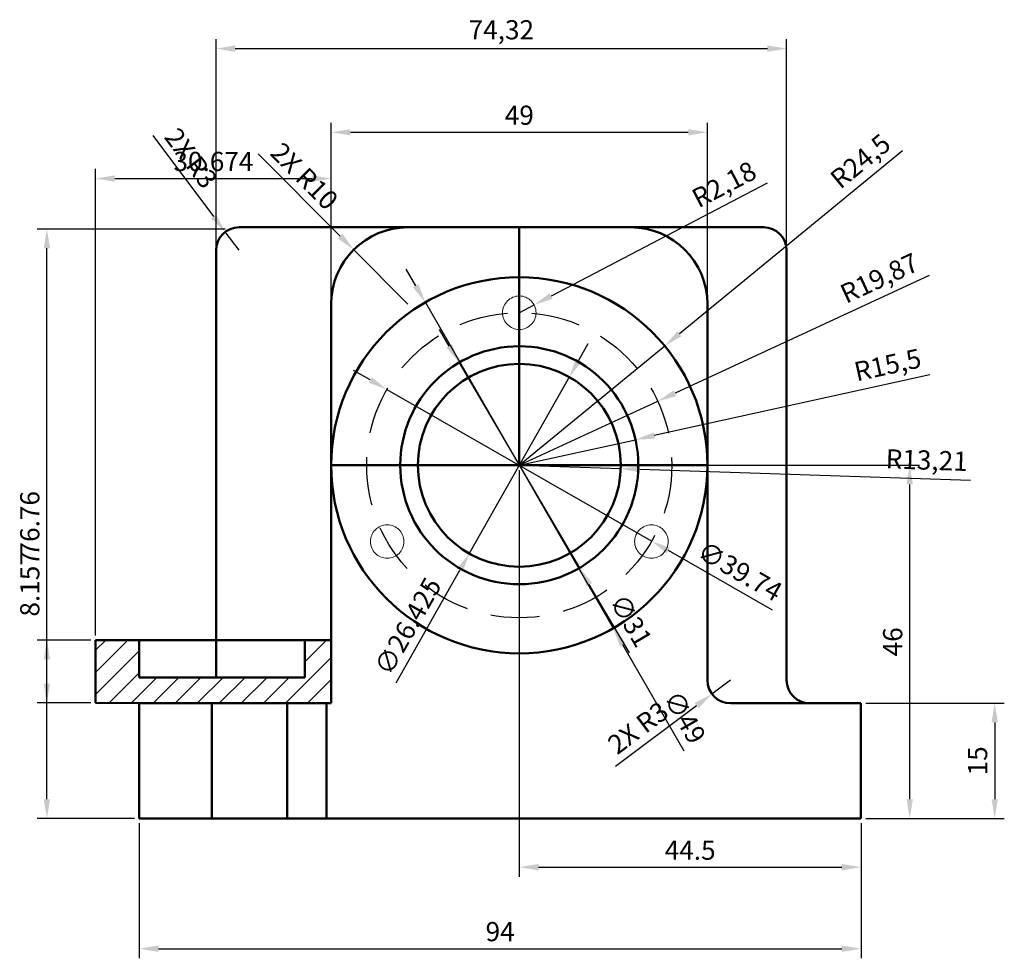
# Model space of a CAD drawing. Units: millimetres. Extents: x 1381 to 2009, y 1325 to 1613.
# Tile 5 of 6: x 1622 to 1750, y 1491 to 1613. Entities that reach past the tile are written whole.
import ezdxf

# ---------------------------------------------------------------- set-up
doc = ezdxf.new("R2010")
doc.units = ezdxf.units.MM
doc.linetypes.add('CENTER', pattern=[50.8, 31.75, -6.35, 6.35, -6.35])
doc.linetypes.add('HIDDEN', pattern=[9.525, 6.35, -3.175])
for name, color, linetype, lineweight in [('M-CNTR', 1, 'CENTER', 18), ('M-DIMS', 2, 'Continuous', 25), ('M-HATC', 8, 'Continuous', 18), ('M-HIDN', 6, 'HIDDEN', 25), ('M-OUTL', 7, 'Continuous', 50)]:
    doc.layers.add(name, color=color, linetype=linetype, lineweight=lineweight)
doc.styles.get("Standard").update_dxf_attribs({"font": 'arial.ttf'})
doc.dimstyles.new('ISO-25', dxfattribs={"dimtxt": 2.5, "dimasz": 2.5, "dimexe": 1.25, "dimexo": 0.625, "dimtad": 1, "dimtxsty": 'Standard', "dimcen": 2.5, "dimadec": 0, "dimazin": 0, "dimtfac": 1, "dimtmove": 0, "dimatfit": 3, "dimfxl": 1, "dimarcsym": 0})

# ---------------------------------------------------------------- blocks, each defined once
blk = doc.blocks.new('*U10')
blk.add_circle((0, 0), 2.18)
blk = doc.blocks.new('*U11')
at = {"layer": 'M-CNTR', "color": 0, "linetype": 'ByBlock', "lineweight": -2, "transparency": 16777216}
blk.add_blockref('*U10', (1686.87, 1575.09), dxfattribs=at)
for p, rotation in [((1669.66, 1545.28), 120), ((1704.07, 1545.28), 240)]:
    blk.add_blockref('*U10', p, dxfattribs=dict(at, rotation=rotation))
blk = doc.blocks.new('*D59')
at = {"layer": 'Defpoints', "color": 0, "transparency": 16777216}
for p in [(1637.37, 1509.22), (1731.37, 1509.22), (1731.37, 1492.25)]:
    blk.add_point(p, dxfattribs=at)
at = {"layer": 'M-DIMS', "color": 0, "lineweight": -2, "transparency": 16777216}
for p, q in [((1637.37, 1508.59), (1637.37, 1491)), ((1731.37, 1508.59), (1731.37, 1491)), ((1639.87, 1492.25), (1728.87, 1492.25))]:
    blk.add_line(p, q, dxfattribs=at)
at = {"layer": 'M-DIMS', "color": 0, "transparency": 16777216}
for points in [[(1639.87, 1492.67), (1639.87, 1491.83), (1637.37, 1492.25)], [(1728.87, 1492.67), (1728.87, 1491.83), (1731.37, 1492.25)]]:
    blk.add_solid(points, dxfattribs=at)
at = {"layer": 'M-DIMS', "color": 0, "transparency": 16777216, "insert": (1684.37, 1494.15), "char_height": 2.5, "attachment_point": 5}
blk.add_mtext('94', dxfattribs=at)
blk = doc.blocks.new('*D60')
at = {"layer": 'Defpoints', "color": 0, "transparency": 16777216}
for p in [(1731.37, 1524.22), (1731.37, 1509.22), (1748.78, 1509.22)]:
    blk.add_point(p, dxfattribs=at)
at = {"layer": 'M-DIMS', "color": 0, "lineweight": -2, "transparency": 16777216}
for p, q in [((1731.99, 1524.22), (1750.03, 1524.22)), ((1748.78, 1521.72), (1748.78, 1511.72)), ((1731.99, 1509.22), (1750.03, 1509.22))]:
    blk.add_line(p, q, dxfattribs=at)
at = {"layer": 'M-DIMS', "color": 0, "transparency": 16777216}
for points in [[(1748.37, 1521.72), (1749.2, 1521.72), (1748.78, 1524.22)], [(1748.37, 1511.72), (1749.2, 1511.72), (1748.78, 1509.22)]]:
    blk.add_solid(points, dxfattribs=at)
at = {"layer": 'M-DIMS', "color": 0, "transparency": 16777216, "insert": (1746.88, 1516.72), "char_height": 2.5, "attachment_point": 5, "rotation": 90}
blk.add_mtext('15', dxfattribs=at)
blk = doc.blocks.new('*D61')
at = {"layer": 'Defpoints', "color": 0, "transparency": 16777216}
for p in [(1721.68, 1609.49), (1647.37, 1583.22), (1721.68, 1583.22)]:
    blk.add_point(p, dxfattribs=at)
at = {"layer": 'M-DIMS', "color": 0, "lineweight": -2, "transparency": 16777216}
for p, q in [((1647.37, 1583.84), (1647.37, 1610.74)), ((1721.68, 1583.84), (1721.68, 1610.74)), ((1649.87, 1609.49), (1719.18, 1609.49))]:
    blk.add_line(p, q, dxfattribs=at)
at = {"layer": 'M-DIMS', "color": 0, "transparency": 16777216}
for points in [[(1649.87, 1609.91), (1649.87, 1609.07), (1647.37, 1609.49)], [(1719.18, 1609.91), (1719.18, 1609.07), (1721.68, 1609.49)]]:
    blk.add_solid(points, dxfattribs=at)
at = {"layer": 'M-DIMS', "color": 0, "transparency": 16777216, "insert": (1684.53, 1611.62), "char_height": 2.5, "attachment_point": 5}
blk.add_mtext('74,32', dxfattribs=at)
blk = doc.blocks.new('*D62')
at = {"layer": 'Defpoints', "color": 0, "transparency": 16777216}
for p in [(1711.37, 1598.59), (1662.37, 1576.22), (1711.37, 1576.22)]:
    blk.add_point(p, dxfattribs=at)
at = {"layer": 'M-DIMS', "color": 0, "lineweight": -2, "transparency": 16777216}
for p, q in [((1662.37, 1576.84), (1662.37, 1599.84)), ((1711.37, 1576.84), (1711.37, 1599.84)), ((1664.87, 1598.59), (1708.87, 1598.59))]:
    blk.add_line(p, q, dxfattribs=at)
at = {"layer": 'M-DIMS', "color": 0, "transparency": 16777216}
for points in [[(1664.87, 1599.01), (1664.87, 1598.18), (1662.37, 1598.59)], [(1708.87, 1599.01), (1708.87, 1598.18), (1711.37, 1598.59)]]:
    blk.add_solid(points, dxfattribs=at)
at = {"layer": 'M-DIMS', "color": 0, "transparency": 16777216, "insert": (1686.87, 1600.49), "char_height": 2.5, "attachment_point": 5}
blk.add_mtext('49', dxfattribs=at)
blk = doc.blocks.new('*D63')
at = {"layer": 'Defpoints', "color": 0, "transparency": 16777216}
for p in [(1705.8, 1570.76), (1686.87, 1555.22)]:
    blk.add_point(p, dxfattribs=at)
at = {"layer": 'M-DIMS', "color": 0, "lineweight": -2, "transparency": 16777216}
for p, q in [((1736.76, 1596.17), (1707.74, 1572.35)), ((1686.87, 1555.22), (1705.8, 1570.76))]:
    blk.add_line(p, q, dxfattribs=at)
at = {"layer": 'M-DIMS', "color": 0, "transparency": 16777216}
blk.add_solid([(1707.47, 1572.67), (1708, 1572.03), (1705.8, 1570.76)], dxfattribs=at)
at = {"layer": 'M-DIMS', "color": 0, "transparency": 16777216, "insert": (1731.49, 1594.59), "char_height": 2.5, "attachment_point": 5, "rotation": 39.3795}
blk.add_mtext('R24,5', dxfattribs=at)
blk = doc.blocks.new('*D64')
at = {"layer": 'Defpoints', "color": 0, "transparency": 16777216}
for p in [(1704.9, 1563.56), (1686.87, 1555.22)]:
    blk.add_point(p, dxfattribs=at)
at = {"layer": 'M-DIMS', "color": 0, "lineweight": -2, "transparency": 16777216}
for p, q in [((1740.26, 1579.92), (1707.17, 1564.61)), ((1686.87, 1555.22), (1704.9, 1563.56))]:
    blk.add_line(p, q, dxfattribs=at)
at = {"layer": 'M-DIMS', "color": 0, "transparency": 16777216}
blk.add_solid([(1706.99, 1564.99), (1707.34, 1564.23), (1704.9, 1563.56)], dxfattribs=at)
at = {"layer": 'M-DIMS', "color": 0, "transparency": 16777216, "insert": (1733.89, 1579.31), "char_height": 2.5, "attachment_point": 5, "rotation": 24.8223}
blk.add_mtext('R19,87', dxfattribs=at)
blk = doc.blocks.new('*D65')
at = {"layer": 'Defpoints', "color": 0, "transparency": 16777216}
for p in [(1702, 1558.55), (1686.87, 1555.22)]:
    blk.add_point(p, dxfattribs=at)
at = {"layer": 'M-DIMS', "color": 0, "lineweight": -2, "transparency": 16777216}
for p, q in [((1740.33, 1566.99), (1704.45, 1559.09)), ((1686.87, 1555.22), (1702, 1558.55))]:
    blk.add_line(p, q, dxfattribs=at)
at = {"layer": 'M-DIMS', "color": 0, "transparency": 16777216}
blk.add_solid([(1704.36, 1559.5), (1704.54, 1558.68), (1702, 1558.55)], dxfattribs=at)
at = {"layer": 'M-DIMS', "color": 0, "transparency": 16777216, "insert": (1734.91, 1567.98), "char_height": 2.5, "attachment_point": 5, "rotation": 12.4201}
blk.add_mtext('R15,5', dxfattribs=at)
blk = doc.blocks.new('*D66')
at = {"layer": 'Defpoints', "color": 0, "transparency": 16777216}
for p in [(1686.87, 1555.22), (1700.07, 1554.78)]:
    blk.add_point(p, dxfattribs=at)
at = {"layer": 'M-DIMS', "color": 0, "lineweight": -2, "transparency": 16777216}
for p, q in [((1686.87, 1555.22), (1700.07, 1554.78)), ((1745.64, 1553.25), (1702.57, 1554.69))]:
    blk.add_line(p, q, dxfattribs=at)
at = {"layer": 'M-DIMS', "color": 0, "transparency": 16777216}
blk.add_solid([(1702.59, 1555.11), (1702.56, 1554.28), (1700.07, 1554.78)], dxfattribs=at)
at = {"layer": 'M-DIMS', "color": 0, "transparency": 16777216, "insert": (1739.92, 1555.57), "char_height": 2.5, "attachment_point": 5, "rotation": 358.0829}
blk.add_mtext('R13,21', dxfattribs=at)
blk = doc.blocks.new('*D67')
at = {"layer": 'Defpoints', "color": 0, "transparency": 16777216}
for p in [(1688.8, 1576.1), (1686.87, 1575.09)]:
    blk.add_point(p, dxfattribs=at)
at = {"layer": 'M-DIMS', "color": 0, "lineweight": -2, "transparency": 16777216}
for p, q in [((1719.16, 1591.98), (1691.02, 1577.26)), ((1686.87, 1575.09), (1688.8, 1576.1))]:
    blk.add_line(p, q, dxfattribs=at)
at = {"layer": 'M-DIMS', "color": 0, "transparency": 16777216}
blk.add_solid([(1690.82, 1577.63), (1691.21, 1576.89), (1688.8, 1576.1)], dxfattribs=at)
at = {"layer": 'M-DIMS', "color": 0, "transparency": 16777216, "insert": (1713.68, 1591.52), "char_height": 2.5, "attachment_point": 5, "rotation": 27.618}
blk.add_mtext('R2,18', dxfattribs=at)
blk = doc.blocks.new('*D83')
at = {"layer": 'Defpoints', "color": 0, "transparency": 16777216}
for p in [(1625.34, 1585.98), (1649.2, 1585.98), (1637.37, 1509.22)]:
    blk.add_point(p, dxfattribs=at)
at = {"layer": 'M-DIMS', "color": 0, "lineweight": -2, "transparency": 16777216}
for p, q in [((1648.57, 1585.98), (1624.09, 1585.98)), ((1625.34, 1511.72), (1625.34, 1583.48)), ((1636.74, 1509.22), (1624.09, 1509.22))]:
    blk.add_line(p, q, dxfattribs=at)
at = {"layer": 'M-DIMS', "color": 0, "transparency": 16777216}
for points in [[(1624.93, 1583.48), (1625.76, 1583.48), (1625.34, 1585.98)], [(1624.93, 1511.72), (1625.76, 1511.72), (1625.34, 1509.22)]]:
    blk.add_solid(points, dxfattribs=at)
at = {"layer": 'M-DIMS', "color": 0, "transparency": 16777216, "insert": (1623.44, 1547.6), "char_height": 2.5, "attachment_point": 5, "rotation": 90}
blk.add_mtext('76.76', dxfattribs=at)
blk = doc.blocks.new('*D84')
at = {"layer": 'Defpoints', "color": 0, "transparency": 16777216}
for p in [(1686.87, 1555.22), (1737.72, 1555.22), (1731.37, 1509.22)]:
    blk.add_point(p, dxfattribs=at)
at = {"layer": 'M-DIMS', "color": 0, "lineweight": -2, "transparency": 16777216}
for p, q in [((1687.49, 1555.22), (1738.97, 1555.22)), ((1737.72, 1511.72), (1737.72, 1552.72)), ((1731.99, 1509.22), (1738.97, 1509.22))]:
    blk.add_line(p, q, dxfattribs=at)
at = {"layer": 'M-DIMS', "color": 0, "transparency": 16777216}
for points in [[(1737.3, 1552.72), (1738.13, 1552.72), (1737.72, 1555.22)], [(1737.3, 1511.72), (1738.13, 1511.72), (1737.72, 1509.22)]]:
    blk.add_solid(points, dxfattribs=at)
at = {"layer": 'M-DIMS', "color": 0, "transparency": 16777216, "insert": (1735.82, 1532.22), "char_height": 2.5, "attachment_point": 5, "rotation": 90}
blk.add_mtext('46', dxfattribs=at)
blk = doc.blocks.new('*D85')
at = {"layer": 'Defpoints', "color": 0, "transparency": 16777216}
for p in [(1686.87, 1555.22), (1731.37, 1509.22), (1731.37, 1502.87)]:
    blk.add_point(p, dxfattribs=at)
at = {"layer": 'M-DIMS', "color": 0, "lineweight": -2, "transparency": 16777216}
for p, q in [((1686.87, 1554.59), (1686.87, 1501.62)), ((1731.37, 1508.59), (1731.37, 1501.62)), ((1689.37, 1502.87), (1728.87, 1502.87))]:
    blk.add_line(p, q, dxfattribs=at)
at = {"layer": 'M-DIMS', "color": 0, "transparency": 16777216}
for points in [[(1689.37, 1503.28), (1689.37, 1502.45), (1686.87, 1502.87)], [(1728.87, 1503.28), (1728.87, 1502.45), (1731.37, 1502.87)]]:
    blk.add_solid(points, dxfattribs=at)
at = {"layer": 'M-DIMS', "color": 0, "transparency": 16777216, "insert": (1709.12, 1504.76), "char_height": 2.5, "attachment_point": 5}
blk.add_mtext('44.5', dxfattribs=at)
blk = doc.blocks.new('*D86')
at = {"layer": 'Defpoints', "color": 0, "transparency": 16777216}
for p in [(1625.34, 1532.43), (1631.69, 1532.43), (1631.69, 1524.27)]:
    blk.add_point(p, dxfattribs=at)
at = {"layer": 'M-DIMS', "color": 0, "lineweight": -2, "transparency": 16777216}
for p, q in [((1625.34, 1532.43), (1625.34, 1544.62)), ((1631.07, 1532.43), (1624.09, 1532.43)), ((1625.34, 1526.77), (1625.34, 1529.93)), ((1631.07, 1524.27), (1624.09, 1524.27))]:
    blk.add_line(p, q, dxfattribs=at)
at = {"layer": 'M-DIMS', "color": 0, "transparency": 16777216}
for points in [[(1624.93, 1529.93), (1625.76, 1529.93), (1625.34, 1532.43)], [(1624.93, 1526.77), (1625.76, 1526.77), (1625.34, 1524.27)]]:
    blk.add_solid(points, dxfattribs=at)
at = {"layer": 'M-DIMS', "color": 0, "transparency": 16777216, "insert": (1623.44, 1539.77), "char_height": 2.5, "attachment_point": 5, "rotation": 90}
blk.add_mtext('8.157', dxfattribs=at)
blk = doc.blocks.new('*D87')
at = {"layer": 'Defpoints', "color": 0, "transparency": 16777216}
for p in [(1662.37, 1592.57), (1631.69, 1532.43), (1662.37, 1532.43)]:
    blk.add_point(p, dxfattribs=at)
at = {"layer": 'M-DIMS', "color": 0, "lineweight": -2, "transparency": 16777216}
for p, q in [((1631.69, 1533.05), (1631.69, 1593.82)), ((1662.37, 1533.05), (1662.37, 1593.82)), ((1634.19, 1592.57), (1659.87, 1592.57))]:
    blk.add_line(p, q, dxfattribs=at)
at = {"layer": 'M-DIMS', "color": 0, "transparency": 16777216}
for points in [[(1634.19, 1592.98), (1634.19, 1592.15), (1631.69, 1592.57)], [(1659.87, 1592.98), (1659.87, 1592.15), (1662.37, 1592.57)]]:
    blk.add_solid(points, dxfattribs=at)
at = {"layer": 'M-DIMS', "color": 0, "transparency": 16777216, "insert": (1647.03, 1594.47), "char_height": 2.5, "attachment_point": 5}
blk.add_mtext('30.674', dxfattribs=at)
blk = doc.blocks.new('*D107')
at = {"layer": 'Defpoints', "color": 0, "transparency": 16777216}
for p in [(1674.63, 1576.44), (1699.1, 1533.99)]:
    blk.add_point(p, dxfattribs=at)
at = {"layer": 'M-DIMS', "color": 0, "lineweight": -2, "transparency": 16777216}
for p, q in [((1673.38, 1578.61), (1672.13, 1580.77)), ((1674.63, 1576.44), (1699.1, 1533.99)), ((1708.33, 1517.98), (1700.35, 1531.83))]:
    blk.add_line(p, q, dxfattribs=at)
at = {"layer": 'M-DIMS', "color": 0, "transparency": 16777216}
for points in [[(1673.74, 1578.82), (1673.02, 1578.4), (1674.63, 1576.44)], [(1700.71, 1532.04), (1699.99, 1531.62), (1699.1, 1533.99)]]:
    blk.add_solid(points, dxfattribs=at)
at = {"layer": 'M-DIMS', "color": 0, "transparency": 16777216, "insert": (1708.15, 1522.24), "char_height": 2.5, "attachment_point": 5, "rotation": 299.9643}
blk.add_mtext('∅49', dxfattribs=at)
blk = doc.blocks.new('*D108')
at = {"layer": 'Defpoints', "color": 0, "transparency": 16777216}
for p in [(1669.62, 1565.09), (1704.11, 1545.35)]:
    blk.add_point(p, dxfattribs=at)
at = {"layer": 'M-DIMS', "color": 0, "lineweight": -2, "transparency": 16777216}
for p, q in [((1667.45, 1566.33), (1665.28, 1567.57)), ((1669.62, 1565.09), (1704.11, 1545.35)), ((1719.84, 1536.35), (1706.28, 1544.11))]:
    blk.add_line(p, q, dxfattribs=at)
at = {"layer": 'M-DIMS', "color": 0, "transparency": 16777216}
for points in [[(1667.66, 1566.69), (1667.25, 1565.97), (1669.62, 1565.09)], [(1706.49, 1544.47), (1706.08, 1543.75), (1704.11, 1545.35)]]:
    blk.add_solid(points, dxfattribs=at)
at = {"layer": 'M-DIMS', "color": 0, "transparency": 16777216, "insert": (1715.44, 1541.14), "char_height": 2.5, "attachment_point": 5, "rotation": 330.221}
blk.add_mtext('∅39.74', dxfattribs=at)
blk = doc.blocks.new('*D109')
at = {"layer": 'Defpoints', "color": 0, "transparency": 16777216}
for p in [(1679.02, 1568.58), (1694.72, 1541.85)]:
    blk.add_point(p, dxfattribs=at)
at = {"layer": 'M-DIMS', "color": 0, "lineweight": -2, "transparency": 16777216}
for p, q in [((1677.75, 1570.74), (1676.48, 1572.89)), ((1679.02, 1568.58), (1694.72, 1541.85)), ((1701.22, 1530.79), (1695.98, 1539.7))]:
    blk.add_line(p, q, dxfattribs=at)
at = {"layer": 'M-DIMS', "color": 0, "transparency": 16777216}
for points in [[(1678.11, 1570.95), (1677.39, 1570.53), (1679.02, 1568.58)], [(1696.34, 1539.91), (1695.63, 1539.49), (1694.72, 1541.85)]]:
    blk.add_solid(points, dxfattribs=at)
at = {"layer": 'M-DIMS', "color": 0, "transparency": 16777216, "insert": (1701.13, 1534.83), "char_height": 2.5, "attachment_point": 5, "rotation": 300.4327}
blk.add_mtext('∅31', dxfattribs=at)
blk = doc.blocks.new('*D110')
at = {"layer": 'Defpoints', "color": 0, "transparency": 16777216}
for p in [(1693.38, 1566.71), (1680.36, 1543.72)]:
    blk.add_point(p, dxfattribs=at)
at = {"layer": 'M-DIMS', "color": 0, "lineweight": -2, "transparency": 16777216}
for p, q in [((1694.61, 1568.89), (1695.84, 1571.07)), ((1693.38, 1566.71), (1680.36, 1543.72)), ((1670.81, 1526.87), (1679.12, 1541.55))]:
    blk.add_line(p, q, dxfattribs=at)
at = {"layer": 'M-DIMS', "color": 0, "transparency": 16777216}
for points in [[(1694.25, 1569.1), (1694.97, 1568.68), (1693.38, 1566.71)], [(1678.76, 1541.75), (1679.49, 1541.34), (1680.36, 1543.72)]]:
    blk.add_solid(points, dxfattribs=at)
at = {"layer": 'M-DIMS', "color": 0, "transparency": 16777216, "insert": (1672.64, 1534.09), "char_height": 2.5, "attachment_point": 5, "rotation": 60.472}
blk.add_mtext('∅26.425', dxfattribs=at)
blk = doc.blocks.new('*D111')
at = {"layer": 'Defpoints', "color": 0, "transparency": 16777216}
for p in [(1665.3, 1583.3), (1672.37, 1576.22)]:
    blk.add_point(p, dxfattribs=at)
at = {"layer": 'M-DIMS', "color": 0, "lineweight": -2, "transparency": 16777216}
for p, q in [((1652.85, 1595.78), (1663.54, 1585.07)), ((1672.37, 1576.22), (1665.3, 1583.3))]:
    blk.add_line(p, q, dxfattribs=at)
at = {"layer": 'M-DIMS', "color": 0, "transparency": 16777216}
blk.add_solid([(1663.83, 1585.36), (1663.24, 1584.77), (1665.3, 1583.3)], dxfattribs=at)
at = {"layer": 'M-DIMS', "color": 0, "transparency": 16777216, "insert": (1658.66, 1592.65), "char_height": 2.5, "attachment_point": 5, "rotation": 314.9409}
blk.add_mtext('2X R10', dxfattribs=at)
blk = doc.blocks.new('*D112')
at = {"layer": 'Defpoints', "color": 0, "transparency": 16777216}
for p in [(1648.56, 1585.62), (1650.37, 1583.22)]:
    blk.add_point(p, dxfattribs=at)
at = {"layer": 'M-DIMS', "color": 0, "lineweight": -2, "transparency": 16777216}
for p, q in [((1639.13, 1598.16), (1647.06, 1587.61)), ((1650.37, 1583.22), (1648.56, 1585.62))]:
    blk.add_line(p, q, dxfattribs=at)
at = {"layer": 'M-DIMS', "color": 0, "transparency": 16777216}
blk.add_solid([(1647.39, 1587.86), (1646.73, 1587.36), (1648.56, 1585.62)], dxfattribs=at)
at = {"layer": 'M-DIMS', "color": 0, "transparency": 16777216, "insert": (1643.86, 1595.03), "char_height": 2.5, "attachment_point": 5, "rotation": 306.9449}
blk.add_mtext('2X R3', dxfattribs=at)
blk = doc.blocks.new('*D113')
at = {"layer": 'Defpoints', "color": 0, "transparency": 16777216}
for p in [(1714.37, 1527.22), (1711.96, 1525.42)]:
    blk.add_point(p, dxfattribs=at)
at = {"layer": 'M-DIMS', "color": 0, "lineweight": -2, "transparency": 16777216}
for p, q in [((1714.37, 1527.22), (1711.96, 1525.42)), ((1699.39, 1516.03), (1709.96, 1523.93))]:
    blk.add_line(p, q, dxfattribs=at)
at = {"layer": 'M-DIMS', "color": 0, "transparency": 16777216}
blk.add_solid([(1709.71, 1524.26), (1710.21, 1523.59), (1711.96, 1525.42)], dxfattribs=at)
at = {"layer": 'M-DIMS', "color": 0, "transparency": 16777216, "insert": (1702.53, 1520.76), "char_height": 2.5, "attachment_point": 5, "rotation": 36.743}
blk.add_mtext('2X R3', dxfattribs=at)

msp = doc.modelspace()

# ---------------------------------------------------------------- hatches: boundary and pattern name
at = {"layer": 'M-HATC'}
h = msp.add_hatch(dxfattribs=at)
h.set_pattern_fill('ANSI31', color=256, scale=0.64)
h.paths.add_polyline_path([(1637.3674, 1532.4271), (1631.6931, 1532.4271), (1631.6931, 1524.2706), (1637.3674, 1524.218), (1662.3674, 1524.218), (1662.3674, 1532.4271), (1658.9514, 1532.4271), (1658.9514, 1527.5885), (1637.3674, 1527.5885)])

# ---------------------------------------------------------------- linework, layer by layer
at = {"layer": 'M-HIDN'}
msp.add_circle((1686.8674, 1555.218), 19.8686, dxfattribs=at)
msp.add_circle((1686.8674, 1555.218), 19.8686, dxfattribs=at)
at = {"layer": 'M-OUTL'}
for p, q in [((1662.3674, 1586.218), (1650.3674, 1586.218)), ((1662.3674, 1586.218), (1672.3674, 1586.218)), ((1672.3674, 1586.218), (1701.3674, 1586.218)), ((1686.8674, 1586.218), (1686.8674, 1555.218)), ((1711.3674, 1586.218), (1701.3674, 1586.218)), ((1711.3674, 1586.218), (1718.6837, 1586.218)), ((1647.3674, 1583.218), (1647.3674, 1527.5885)), ((1721.6837, 1583.218), (1721.6837, 1527.218)), ((1662.3674, 1524.218), (1662.3674, 1576.218)), ((1711.3674, 1527.218), (1711.3674, 1576.218)), ((1662.3674, 1555.218), (1711.3674, 1555.218)), ((1637.3674, 1532.4271), (1631.6931, 1532.4271)), ((1631.6931, 1532.4271), (1631.6931, 1524.2706)), ((1637.3674, 1532.4271), (1662.3674, 1532.4271)), ((1637.3674, 1532.4271), (1637.3674, 1527.5885)), ((1658.9514, 1527.5885), (1658.9514, 1532.4271)), ((1637.3674, 1527.5885), (1658.9514, 1527.5885)), ((1631.6931, 1524.2706), (1637.3674, 1524.218)), ((1637.3674, 1509.218), (1637.3674, 1524.218)), ((1637.3674, 1524.218), (1662.3674, 1524.218)), ((1646.8045, 1509.218), (1646.8045, 1524.218)), ((1656.6491, 1524.218), (1656.6491, 1509.218)), ((1661.7627, 1509.218), (1661.7627, 1524.218)), ((1714.3674, 1524.218), (1724.6837, 1524.218)), ((1731.3674, 1524.218), (1724.6837, 1524.218)), ((1731.3674, 1509.218), (1731.3674, 1524.218)), ((1637.3674, 1509.218), (1731.3674, 1509.218))]:
    msp.add_line(p, q, dxfattribs=at)
for radius in [24.5, 15.5, 13.2126]:
    msp.add_circle((1686.8674, 1555.218), radius, dxfattribs=at)
for centre, radius, start, end in [((1650.3674, 1583.218), 3, 90, 180), ((1672.3674, 1576.218), 10, 90, 180), ((1701.3674, 1576.218), 10, 0, 90), ((1718.6837, 1583.218), 3, 0, 90), ((1714.3674, 1527.218), 3, 180, 270), ((1724.6837, 1527.218), 3, 180, 270)]:
    msp.add_arc(centre, radius, start, end, dxfattribs=at)

# ---------------------------------------------------------------- block references
at = {"layer": 'M-CNTR'}
msp.add_blockref('*U11', (0, 0), dxfattribs=at)

# ---------------------------------------------------------------- dimensions: what is measured, and where the dimension line sits
at = {"layer": 'M-DIMS'}
for base, p1, p2, override, picture, middle in [((1721.6837, 1609.4903), (1647.3674, 1583.218), (1721.6837, 1583.218), {"dimclrd": 0, "dimclre": 0, "dimclrt": 0}, '*D61', (1684.5255, 1611.6177)), ((1711.3674, 1598.5926), (1662.3674, 1576.218), (1711.3674, 1576.218), {"dimclrd": 0, "dimclre": 0, "dimclrt": 0}, '*D62', (1686.8674, 1600.494)), ((1662.3674, 1592.568), (1631.6931, 1532.4271), (1662.3674, 1532.4271), {"dimdec": 3, "dimlfac": 1, "dimrnd": 0, "dimzin": 0, "dimdsep": 46, "dimlunit": 2}, '*D87', (1647.0302, 1594.4703)), ((1731.3674, 1502.868), (1686.8674, 1555.218), (1731.3674, 1509.218), {"dimdec": 1, "dimlfac": 1, "dimrnd": 0, "dimzin": 0, "dimdsep": 46, "dimlunit": 2}, '*D85', (1709.1174, 1504.7644)), ((1731.3674, 1492.2484), (1637.3674, 1509.218), (1731.3674, 1509.218), {"dimclrd": 0, "dimclre": 0, "dimclrt": 0}, '*D59', (1684.3674, 1494.1499))]:
    dim = msp.add_linear_dim(base=base, p1=p1, p2=p2, dimstyle='ISO-25', override=override, dxfattribs=at)
    dim.commit()
    dim.dimension.update_dxf_attribs({"geometry": picture, "text_midpoint": middle})
for center, mpoint, picture, middle in [((1650.3674, 1583.218), (1648.5642, 1585.6157), '*D112', (1643.865, 1595.0292)), ((1672.3674, 1576.218), (1665.3036, 1583.2964), '*D111', (1658.657, 1592.6485)), ((1714.3674, 1527.218), (1711.9634, 1525.4234), '*D113', (1702.5334, 1520.7573))]:
    dim = msp.add_radius_dim(center=center, mpoint=mpoint, text='2X <>', dimstyle='ISO-25', override={"dimdec": 0, "dimlfac": 1, "dimrnd": 0, "dimzin": 0, "dimdsep": 46, "dimlunit": 2}, dxfattribs=at)
    dim.commit()
    dim.dimension.update_dxf_attribs({"geometry": picture, "text_midpoint": middle})
for center, mpoint, picture, middle in [((1686.8674, 1555.218), (1705.8049, 1570.7622), '*D63', (1732.8354, 1592.9491)), ((1686.8674, 1575.0867), (1688.8028, 1576.0993), '*D67', (1714.6668, 1589.631)), ((1686.8674, 1555.218), (1704.9004, 1563.559), '*D64', (1734.7832, 1577.3809)), ((1686.8674, 1555.218), (1702.0046, 1558.5517), '*D65', (1735.3675, 1565.8993)), ((1686.8674, 1555.218), (1700.0726, 1554.776), '*D66', (1739.8473, 1553.4447))]:
    dim = msp.add_radius_dim(center=center, mpoint=mpoint, dimstyle='ISO-25', override={"dimclrd": 0, "dimclre": 0, "dimclrt": 0}, dxfattribs=at)
    dim.commit()
    dim.dimension.update_dxf_attribs({"geometry": picture, "text_midpoint": middle, "dimtype": 164})
for base, p1, p2, override, picture, middle in [((1625.3431, 1585.9823), (1637.3674, 1509.218), (1649.1996, 1585.9823), {"dimdec": 2, "dimlfac": 1, "dimrnd": 0, "dimzin": 0, "dimdsep": 46, "dimlunit": 2}, '*D83', (1623.4417, 1547.6002)), ((1737.7174, 1555.218), (1731.3674, 1509.218), (1686.8674, 1555.218), {"dimdec": 0, "dimlfac": 1, "dimrnd": 0, "dimzin": 0, "dimdsep": 46, "dimlunit": 2}, '*D84', (1735.8159, 1532.218)), ((1625.34309, 1532.4271), (1631.69309, 1524.27057), (1631.69309, 1532.4271), {"dimdec": 3, "dimlfac": 1, "dimrnd": 0, "dimzin": 0, "dimdsep": 46, "dimlunit": 2}, '*D86', (1623.44165, 1539.77191)), ((1748.783, 1509.218), (1731.3674, 1524.218), (1731.3674, 1509.218), {"dimclrd": 0, "dimclre": 0, "dimclrt": 0}, '*D60', (1746.8815, 1516.718))]:
    dim = msp.add_linear_dim(base=base, p1=p1, p2=p2, angle=90, dimstyle='ISO-25', override=override, dxfattribs=at)
    dim.commit()
    dim.dimension.update_dxf_attribs({"geometry": picture, "text_midpoint": middle})
for p1, p2, override, picture, middle in [((1674.6306, 1576.4433), (1699.1042, 1533.9928), {"dimdec": 0, "dimlfac": 1, "dimrnd": 0, "dimzin": 0, "dimdsep": 46, "dimlunit": 2}, '*D107', (1706.4462, 1521.2576)), ((1679.0162, 1568.5825), (1694.7185, 1541.8536), {"dimdec": 0, "dimlfac": 1, "dimrnd": 0, "dimzin": 0, "dimdsep": 46, "dimlunit": 2}, '*D109', (1699.4292, 1533.8349)), ((1669.6224, 1565.0859), (1704.1123, 1545.3502), {"dimdec": 2, "dimlfac": 1, "dimrnd": 0, "dimzin": 0, "dimdsep": 46, "dimlunit": 2}, '*D108', (1714.4593, 1539.4295))]:
    dim = msp.add_diameter_dim_2p(p1=p1, p2=p2, dimstyle='ISO-25', override=override, dxfattribs=at)
    dim.commit()
    dim.dimension.update_dxf_attribs({"geometry": picture, "text_midpoint": middle, "dimtype": 163})
dim = msp.add_diameter_dim_2p(p1=(1693.3792, 1566.7145), p2=(1680.3556, 1543.7216), dimstyle='ISO-25', override={"dimdec": 3, "dimlfac": 1, "dimrnd": 0, "dimzin": 0, "dimdsep": 46, "dimlunit": 2}, dxfattribs=at)
dim.commit()
dim.dimension.update_dxf_attribs({"geometry": '*D110', "text_midpoint": (1674.3509, 1533.1204)})

doc.saveas('drawing.dxf')
